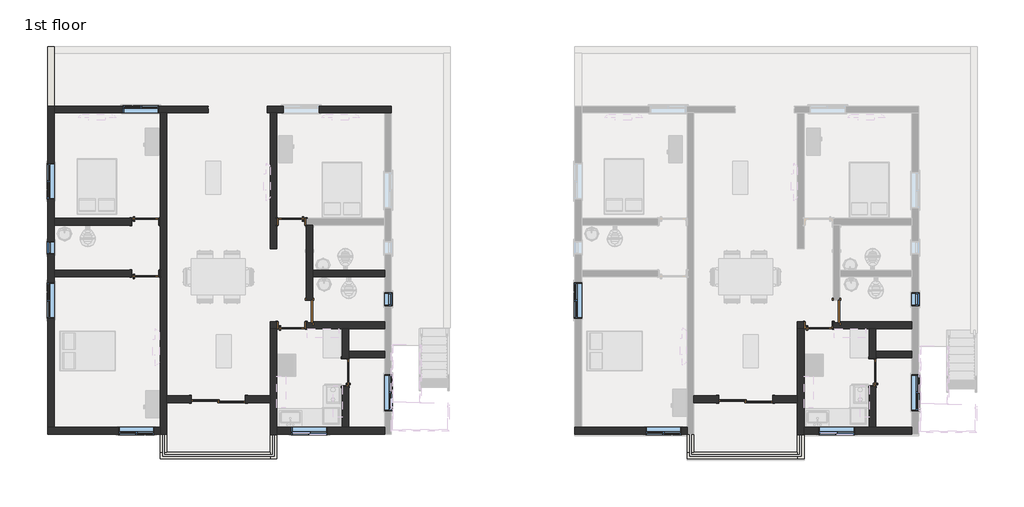
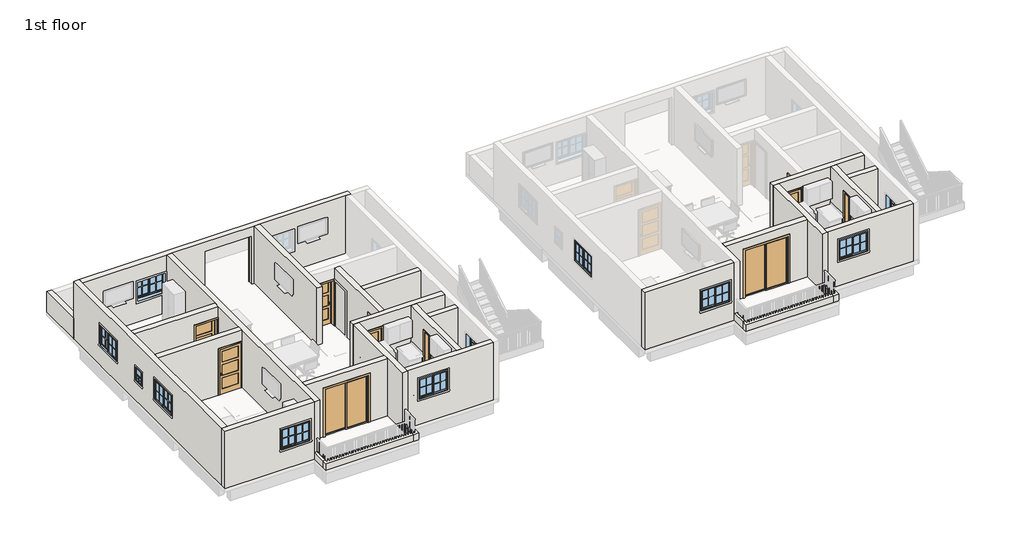
# One storey, part 1 of 8: 30 walls, 13 windows, 11 doors.
"""IFC4 building model written with IfcOpenShell, lengths in millimetres."""

from ifc_helpers import new_model, si_unit, frame, origin, place, context, project, spatial, polyline, outline, extrude, faceted_brep, transform, mapped, element, save
from components import door_d4d75d1e, door_2334f446, door_80766924, door_a1484949, window_608ea798, window_2eef0573, window_a5b1ea32

model = new_model("IFC4")

# Units and contexts
model_context = context("Model", 3, world=origin())
ifc_project = project(units=[si_unit("LENGTHUNIT", "METRE", prefix="MILLI")], contexts=[model_context])

# Site, building, storey
site = spatial("IfcSite", under=ifc_project)
building = spatial("IfcBuilding", under=site)
storey = spatial("IfcBuildingStorey", under=building, Name="1st floor", Elevation=3810.0)

# Doors
placement = place(None, origin())
door_shape = door_d4d75d1e(model_context)
element("IfcDoor", 1, ObjectType="Door-Double-Sliding : 72\" x 84\"", at=placement, inside=storey, context=model_context, shape_type="MappedRepresentation", body=[
    mapped(door_shape, transform((-10509.3993763, -3297.2064015, 3810.0), x_axis=(-1.0, 0.0, 0.0), y_axis=(0.0, -1.0, 0.0), z_axis=(0.0, 0.0, 1.0))),
])
element("IfcDoor", 2, ObjectType="Door-Double-Sliding : 72\" x 84\"", at=placement, inside=storey, context=model_context, shape_type="MappedRepresentation", body=[
    mapped(door_shape, transform((7365.1761273, -3297.2064015, 3810.0), x_axis=(-1.0, 0.0, 0.0), y_axis=(0.0, -1.0, 0.0), z_axis=(0.0, 0.0, 1.0))),
])
door_2_shape = door_2334f446(model_context)
element("IfcDoor", 3, ObjectType="Door-Interior-Single-3_Panel_Vert-Wood : 36\" x 80\"", at=placement, inside=storey, context=model_context, shape_type="MappedRepresentation", body=[
    mapped(door_2_shape, transform((-12985.8993763, 2598.7685985, 3810.0), x_axis=(1.0, 0.0, 0.0), y_axis=(0.0, 1.0, 0.0), z_axis=(0.0, 0.0, 1.0))),
])
door_3_shape = door_80766924(model_context)
element("IfcDoor", 4, ObjectType="Door-Interior-Single-3_Panel_Vert-Wood : 36\" x 80\"", at=placement, inside=storey, context=model_context, shape_type="MappedRepresentation", body=[
    mapped(door_3_shape, transform((-12985.8993763, 839.8185985, 3810.0), x_axis=(1.0, 0.0, 0.0), y_axis=(0.0, 1.0, 0.0), z_axis=(0.0, 0.0, 1.0))),
])
element("IfcDoor", 5, ObjectType="Door-Interior-Single-3_Panel_Vert-Wood : 36\" x 80\"", at=placement, inside=storey, context=model_context, shape_type="MappedRepresentation", body=[
    mapped(door_3_shape, transform((-6200.9243763, -2509.8064015, 3810.0), x_axis=(0.0, 1.0, 0.0), y_axis=(-1.0, 0.0, 0.0), z_axis=(0.0, 0.0, 1.0))),
])
element("IfcDoor", 6, ObjectType="Door-Interior-Single-3_Panel_Vert-Wood : 36\" x 80\"", at=placement, inside=storey, context=model_context, shape_type="MappedRepresentation", body=[
    mapped(door_3_shape, transform((-8032.8993763, -912.7814015, 3810.0), x_axis=(1.0, 0.0, 0.0), y_axis=(0.0, 1.0, 0.0), z_axis=(0.0, 0.0, 1.0))),
])
element("IfcDoor", 7, ObjectType="Door-Interior-Single-3_Panel_Vert-Wood : 36\" x 80\"", at=placement, inside=storey, context=model_context, shape_type="MappedRepresentation", body=[
    mapped(door_3_shape, transform((-8032.8993763, 2598.7685985, 3810.0), x_axis=(-1.0, 0.0, 0.0), y_axis=(0.0, -1.0, 0.0), z_axis=(0.0, 0.0, 1.0))),
])
element("IfcDoor", 8, ObjectType="Door-Interior-Single-3_Panel_Vert-Wood : 36\" x 80\"", at=placement, inside=storey, context=model_context, shape_type="MappedRepresentation", body=[
    mapped(door_3_shape, transform((11673.6511273, -2509.8064015, 3810.0), x_axis=(0.0, 1.0, 0.0), y_axis=(-1.0, 0.0, 0.0), z_axis=(0.0, 0.0, 1.0))),
])
element("IfcDoor", 9, ObjectType="Door-Interior-Single-3_Panel_Vert-Wood : 36\" x 80\"", at=placement, inside=storey, context=model_context, shape_type="MappedRepresentation", body=[
    mapped(door_3_shape, transform((9841.6761273, -912.7814015, 3810.0), x_axis=(1.0, 0.0, 0.0), y_axis=(0.0, 1.0, 0.0), z_axis=(0.0, 0.0, 1.0))),
])
door_4_shape = door_a1484949(model_context)
element("IfcDoor", 10, ObjectType="Single-Flush : 30\" x 80\"", at=placement, inside=storey, context=model_context, shape_type="MappedRepresentation", body=[
    mapped(door_4_shape, transform((-7423.2993763, -452.4064015, 3810.0), x_axis=(0.0, -1.0, 0.0), y_axis=(1.0, 0.0, 0.0), z_axis=(0.0, 0.0, 1.0))),
])
element("IfcDoor", 11, ObjectType="Single-Flush : 30\" x 80\"", at=placement, inside=storey, context=model_context, shape_type="MappedRepresentation", body=[
    mapped(door_4_shape, transform((10451.2761273, -452.4064015, 3810.0), x_axis=(0.0, -1.0, 0.0), y_axis=(1.0, 0.0, 0.0), z_axis=(0.0, 0.0, 1.0))),
])

# Walls
element("IfcWall", 12, at=placement, inside=storey, context=model_context, shape_type="Brep", body=[
    faceted_brep([(-16300.5993763, 6519.8935985, 3810.0), (-16300.5993763, -4376.7064015, 3810.0), (-16300.5993763, -4376.7064015, 6400.8), (-16300.5993763, 6519.8935985, 6400.8), (-16300.5993763, 4576.7935985, 5638.8), (-16300.5993763, 3357.5935985, 5638.8), (-16300.5993763, 3357.5935985, 4724.4), (-16300.5993763, 4576.7935985, 4724.4), (-16300.5993763, -681.0064015, 5638.8), (-16300.5993763, -681.0064015, 4724.4), (-16300.5993763, 538.1935985, 4724.4), (-16300.5993763, 538.1935985, 5638.8), (-16300.5993763, 1935.1935985, 5334.0), (-16300.5993763, 1503.3935985, 5334.0), (-16300.5993763, 1503.3935985, 4724.4), (-16300.5993763, 1935.1935985, 4724.4), (-16071.9993763, 6519.8935985, 3810.0), (-16071.9993763, 6519.8935985, 6400.8), (-16071.9993763, 6291.2935985, 6400.8), (-16071.9993763, 2709.8935985, 6400.8), (-16071.9993763, 2481.2935985, 6400.8), (-16071.9993763, 957.2935985, 6400.8), (-16071.9993763, 728.6935985, 6400.8), (-16071.9993763, -4376.7064015, 6400.8), (-16071.9993763, -4376.7064015, 3810.0), (-16071.9993763, 728.6935985, 3810.0), (-16071.9993763, 957.2935985, 3810.0), (-16071.9993763, 2481.2935985, 3810.0), (-16071.9993763, 2709.8935985, 3810.0), (-16071.9993763, 6291.2935985, 3810.0), (-16071.9993763, 4576.7935985, 5638.8), (-16071.9993763, 4576.7935985, 4724.4), (-16071.9993763, 3357.5935985, 4724.4), (-16071.9993763, 3357.5935985, 5638.8), (-16071.9993763, -681.0064015, 5638.8), (-16071.9993763, 538.1935985, 5638.8), (-16071.9993763, 538.1935985, 4724.4), (-16071.9993763, -681.0064015, 4724.4), (-16071.9993763, 1935.1935985, 5334.0), (-16071.9993763, 1935.1935985, 4724.4), (-16071.9993763, 1503.3935985, 4724.4), (-16071.9993763, 1503.3935985, 5334.0)], [[[0, 1, 2, 3], [4, 5, 6, 7], [8, 9, 10, 11], [12, 13, 14, 15]], [[16, 17, 18, 19, 20, 21, 22, 23, 24, 25, 26, 27, 28, 29], [30, 31, 32, 33], [34, 35, 36, 37], [38, 39, 40, 41]], [[1, 0, 16, 29, 28, 27, 26, 25, 24]], [[3, 2, 23, 22, 21, 20, 19, 18, 17]], [[0, 3, 17, 16]], [[2, 1, 24, 23]], [[31, 30, 4, 7]], [[32, 31, 7, 6]], [[33, 32, 6, 5]], [[30, 33, 5, 4]], [[9, 8, 34, 37]], [[10, 9, 37, 36]], [[11, 10, 36, 35]], [[8, 11, 35, 34]], [[39, 38, 12, 15]], [[40, 39, 15, 14]], [[41, 40, 14, 13]], [[38, 41, 13, 12]]]),
])
element("IfcWall", 13, at=placement, inside=storey, context=model_context, shape_type="SweptSolid", body=[
    extrude(outline(polyline([(6400.8, -12490.5993763), (6400.8, -16071.9993763), (3810.0, -16071.9993763), (3810.0, -13468.4993763), (5867.4, -13468.4993763), (5867.4, -12503.2993763), (3810.0, -12503.2993763), (3810.0, -12490.5993763), (6400.8, -12490.5993763)])), frame((0.0, 2481.2935985, 0.0), z_axis=(0.0, 1.0, 0.0), x_axis=(0.0, 0.0, 1.0)), (0.0, 0.0, 1.0), 228.6),
])
element("IfcWall", 14, at=placement, inside=storey, context=model_context, shape_type="Brep", body=[
    faceted_brep([(-4641.9993763, 6291.2935985, 6400.8), (-4870.5993763, 6291.2935985, 6400.8), (-8528.1993763, 6291.2935985, 6400.8), (-8756.7993763, 6291.2935985, 6400.8), (-12261.9993763, 6291.2935985, 6400.8), (-12490.5993763, 6291.2935985, 6400.8), (-16071.9993763, 6291.2935985, 6400.8), (-16071.9993763, 6291.2935985, 3810.0), (-12490.5993763, 6291.2935985, 3810.0), (-12261.9993763, 6291.2935985, 3810.0), (-10861.6993763, 6291.2935985, 3810.0), (-10861.6993763, 6291.2935985, 5979.5), (-8861.6993763, 6291.2935985, 5979.5), (-8861.6993763, 6291.2935985, 3810.0), (-8756.7993763, 6291.2935985, 3810.0), (-8528.1993763, 6291.2935985, 3810.0), (-4870.5993763, 6291.2935985, 3810.0), (-4641.9993763, 6291.2935985, 3810.0), (-8312.2993763, 6291.2935985, 5638.8), (-7093.0993763, 6291.2935985, 5638.8), (-7093.0993763, 6291.2935985, 4724.4), (-8312.2993763, 6291.2935985, 4724.4), (-12528.6993763, 6291.2935985, 5638.8), (-12528.6993763, 6291.2935985, 4724.4), (-13747.8993763, 6291.2935985, 4724.4), (-13747.8993763, 6291.2935985, 5638.8), (-16071.9993763, 6519.8935985, 6400.8), (-4641.9993763, 6519.8935985, 6400.8), (-4641.9993763, 6519.8935985, 3810.0), (-8861.6993763, 6519.8935985, 3810.0), (-8861.6993763, 6519.8935985, 5979.5), (-10861.6993763, 6519.8935985, 5979.5), (-10861.6993763, 6519.8935985, 3810.0), (-16071.9993763, 6519.8935985, 3810.0), (-8312.2993763, 6519.8935985, 5638.8), (-8312.2993763, 6519.8935985, 4724.4), (-7093.0993763, 6519.8935985, 4724.4), (-7093.0993763, 6519.8935985, 5638.8), (-12528.6993763, 6519.8935985, 5638.8), (-13747.8993763, 6519.8935985, 5638.8), (-13747.8993763, 6519.8935985, 4724.4), (-12528.6993763, 6519.8935985, 4724.4), (-10861.6993763, 6499.8935985, 3810.0), (-10876.6993763, 6499.8935985, 3810.0), (-10876.6993763, 6429.8935985, 3810.0), (-10861.6993763, 6429.8935985, 3810.0), (-8861.6993763, 6429.8935985, 3810.0), (-8846.6993763, 6429.8935985, 3810.0), (-8846.6993763, 6499.8935985, 3810.0), (-8861.6993763, 6499.8935985, 3810.0), (-8861.6993763, 6499.8935985, 5979.5), (-10861.6993763, 6499.8935985, 5979.5), (-10861.6993763, 6429.8935985, 5979.5), (-8861.6993763, 6429.8935985, 5979.5), (-10876.6993763, 6429.8935985, 5994.5), (-8846.6993763, 6429.8935985, 5994.5), (-8846.6993763, 6499.8935985, 5994.5), (-10876.6993763, 6499.8935985, 5994.5)], [[[0, 1, 2, 3, 4, 5, 6, 7, 8, 9, 10, 11, 12, 13, 14, 15, 16, 17], [18, 19, 20, 21], [22, 23, 24, 25]], [[26, 27, 28, 29, 30, 31, 32, 33], [34, 35, 36, 37], [38, 39, 40, 41]], [[7, 33, 32, 42, 43, 44, 45, 10, 9, 8]], [[28, 17, 16, 15, 14, 13, 46, 47, 48, 49, 29]], [[6, 5, 4, 3, 2, 1, 0, 27, 26]], [[7, 6, 26, 33]], [[0, 17, 28, 27]], [[50, 51, 31, 30]], [[52, 53, 12, 11]], [[45, 52, 11, 10]], [[53, 46, 13, 12]], [[53, 52, 45, 44, 54, 55, 47, 46]], [[47, 55, 56, 48]], [[51, 50, 49, 48, 56, 57, 43, 42]], [[49, 50, 30, 29]], [[51, 42, 32, 31]], [[54, 44, 43, 57]], [[55, 54, 57, 56]], [[35, 34, 18, 21]], [[36, 35, 21, 20]], [[37, 36, 20, 19]], [[34, 37, 19, 18]], [[23, 22, 38, 41]], [[24, 23, 41, 40]], [[25, 24, 40, 39]], [[22, 25, 39, 38]]]),
])
element("IfcWall", 15, at=placement, inside=storey, context=model_context, shape_type="Brep", body=[
    faceted_brep([(-4870.5993763, -4376.7064015, 3810.0), (-6089.7993763, -4376.7064015, 3810.0), (-6318.3993763, -4376.7064015, 3810.0), (-8528.1993763, -4376.7064015, 3810.0), (-8528.1993763, -4376.7064015, 6400.8), (-6318.3993763, -4376.7064015, 6400.8), (-6089.7993763, -4376.7064015, 6400.8), (-4870.5993763, -4376.7064015, 6400.8), (-8032.8993763, -4376.7064015, 5867.4), (-8032.8993763, -4376.7064015, 4953.0), (-6813.6993763, -4376.7064015, 4953.0), (-6813.6993763, -4376.7064015, 5867.4), (-4870.5993763, -4605.3064015, 3810.0), (-4870.5993763, -4605.3064015, 6400.8), (-8528.1993763, -4605.3064015, 6400.8), (-8528.1993763, -4605.3064015, 3810.0), (-8032.8993763, -4605.3064015, 5867.4), (-6813.6993763, -4605.3064015, 5867.4), (-6813.6993763, -4605.3064015, 4953.0), (-8032.8993763, -4605.3064015, 4953.0)], [[[0, 1, 2, 3, 4, 5, 6, 7], [8, 9, 10, 11]], [[12, 13, 14, 15], [16, 17, 18, 19]], [[3, 2, 1, 0, 12, 15]], [[7, 6, 5, 4, 14, 13]], [[0, 7, 13, 12]], [[4, 3, 15, 14]], [[9, 8, 16, 19]], [[10, 9, 19, 18]], [[11, 10, 18, 17]], [[8, 11, 17, 16]]]),
])
element("IfcWall", 16, at=placement, inside=storey, context=model_context, shape_type="Brep", body=[
    faceted_brep([(-8756.7993763, 6291.2935985, 3810.0), (-8756.7993763, 1681.1935985, 3810.0), (-8756.7993763, 1681.1935985, 6400.8), (-8756.7993763, 6291.2935985, 6400.8), (-8528.1993763, 6291.2935985, 3810.0), (-8528.1993763, 6291.2935985, 6400.8), (-8528.1993763, 2709.8935985, 6400.8), (-8528.1993763, 2481.2935985, 6400.8), (-8528.1993763, 1681.1935985, 6400.8), (-8528.1993763, 1681.1935985, 3810.0), (-8528.1993763, 2481.2935985, 3810.0), (-8528.1993763, 2709.8935985, 3810.0)], [[[0, 1, 2, 3]], [[4, 5, 6, 7, 8, 9, 10, 11]], [[1, 0, 4, 11, 10, 9]], [[2, 1, 9, 8]], [[3, 2, 8, 7, 6, 5]], [[0, 3, 5, 4]]]),
])
element("IfcWall", 17, at=placement, inside=storey, context=model_context, shape_type="Brep", body=[
    faceted_brep([(-8756.7993763, -5214.9064015, 3810.0), (-12261.9993763, -5214.9064015, 3810.0), (-12490.5993763, -5214.9064015, 3810.0), (-12490.5993763, -5214.9064015, 4114.8), (-12261.9993763, -5214.9064015, 4114.8), (-8756.7993763, -5214.9064015, 4114.8), (-8756.7993763, -5443.5064015, 3810.0), (-8756.7993763, -5443.5064015, 4114.8), (-12490.5993763, -5443.5064015, 4114.8), (-12490.5993763, -5443.5064015, 3810.0)], [[[0, 1, 2, 3, 4, 5]], [[6, 7, 8, 9]], [[2, 1, 0, 6, 9]], [[5, 4, 3, 8, 7]], [[0, 5, 7, 6]], [[3, 2, 9, 8]]]),
])
element("IfcWall", 18, at=placement, inside=storey, context=model_context, shape_type="SweptSolid", body=[
    extrude(outline(polyline([(-12261.9993763, -4611.6564015), (-12261.9993763, -5214.9064015), (-12490.5993763, -5214.9064015), (-12490.5993763, -4611.6564015), (-12261.9993763, -4611.6564015)])), frame((0.0, 0.0, 3810.0), z_axis=(0.0, 0.0, 1.0), x_axis=(1.0, 0.0, 0.0)), (0.0, 0.0, 1.0), 304.8),
])
element("IfcWall", 19, at=placement, inside=storey, context=model_context, shape_type="Brep", body=[
    faceted_brep([(-16300.5993763, -4605.3064015, 3810.0), (-12490.5993763, -4605.3064015, 3810.0), (-12490.5993763, -4605.3064015, 6400.8), (-16300.5993763, -4605.3064015, 6400.8), (-13900.2993763, -4605.3064015, 5638.8), (-12681.0993763, -4605.3064015, 5638.8), (-12681.0993763, -4605.3064015, 4724.4), (-13900.2993763, -4605.3064015, 4724.4), (-16300.5993763, -4376.7064015, 3810.0), (-16300.5993763, -4376.7064015, 6400.8), (-16071.9993763, -4376.7064015, 6400.8), (-12490.5993763, -4376.7064015, 6400.8), (-12490.5993763, -4376.7064015, 3810.0), (-16071.9993763, -4376.7064015, 3810.0), (-13900.2993763, -4376.7064015, 5638.8), (-13900.2993763, -4376.7064015, 4724.4), (-12681.0993763, -4376.7064015, 4724.4), (-12681.0993763, -4376.7064015, 5638.8)], [[[0, 1, 2, 3], [4, 5, 6, 7]], [[8, 9, 10, 11, 12, 13], [14, 15, 16, 17]], [[1, 0, 8, 13, 12]], [[3, 2, 11, 10, 9]], [[0, 3, 9, 8]], [[15, 14, 4, 7]], [[16, 15, 7, 6]], [[17, 16, 6, 5]], [[14, 17, 5, 4]], [[2, 1, 12, 11]]]),
])
element("IfcWall", 20, at=placement, inside=storey, context=model_context, shape_type="SweptSolid", body=[
    extrude(outline(polyline([(3810.0, -12261.9993763), (3810.0, -11423.7993763), (5943.6, -11423.7993763), (5943.6, -9594.9993763), (3810.0, -9594.9993763), (3810.0, -8756.7993763), (6400.8, -8756.7993763), (6400.8, -12261.9993763), (3810.0, -12261.9993763)])), frame((0.0, -3538.5064015, 0.0), z_axis=(0.0, 1.0, 0.0), x_axis=(0.0, 0.0, 1.0)), (0.0, 0.0, 1.0), 228.6),
])
element("IfcWall", 21, at=placement, inside=storey, context=model_context, shape_type="Brep", body=[
    faceted_brep([(-8756.7993763, -795.3064015, 6400.8), (-7537.5993763, -795.3064015, 6400.8), (-7308.9993763, -795.3064015, 6400.8), (-4870.5993763, -795.3064015, 6400.8), (-4870.5993763, -795.3064015, 3810.0), (-7308.9993763, -795.3064015, 3810.0), (-7308.9993763, -795.3064015, 5842.0), (-7537.5993763, -795.3064015, 5842.0), (-7537.5993763, -795.3064015, 3810.0), (-7550.2993763, -795.3064015, 3810.0), (-7550.2993763, -795.3064015, 5867.4), (-8515.4993763, -795.3064015, 5867.4), (-8515.4993763, -795.3064015, 3810.0), (-8756.7993763, -795.3064015, 3810.0), (-4870.5993763, -1023.9064015, 6400.8), (-6089.7993763, -1023.9064015, 6400.8), (-6318.3993763, -1023.9064015, 6400.8), (-8528.1993763, -1023.9064015, 6400.8), (-8756.7993763, -1023.9064015, 6400.8), (-8756.7993763, -1023.9064015, 3810.0), (-8528.1993763, -1023.9064015, 3810.0), (-8515.4993763, -1023.9064015, 3810.0), (-8515.4993763, -1023.9064015, 5867.4), (-7550.2993763, -1023.9064015, 5867.4), (-7550.2993763, -1023.9064015, 3810.0), (-6318.3993763, -1023.9064015, 3810.0), (-6089.7993763, -1023.9064015, 3810.0), (-4870.5993763, -1023.9064015, 3810.0), (-7537.5993763, -833.4064015, 3810.0), (-7308.9993763, -833.4064015, 3810.0), (-7537.5993763, -833.4064015, 5842.0), (-7308.9993763, -833.4064015, 5842.0)], [[[0, 1, 2, 3, 4, 5, 6, 7, 8, 9, 10, 11, 12, 13]], [[14, 15, 16, 17, 18, 19, 20, 21, 22, 23, 24, 25, 26, 27]], [[4, 27, 26, 25, 24, 9, 8, 28, 29, 5]], [[13, 12, 21, 20, 19]], [[3, 2, 1, 0, 18, 17, 16, 15, 14]], [[4, 3, 14, 27]], [[23, 10, 9, 24]], [[10, 23, 22, 11]], [[11, 22, 21, 12]], [[30, 28, 8, 7]], [[29, 31, 6, 5]], [[28, 30, 31, 29]], [[31, 30, 7, 6]], [[0, 13, 19, 18]]]),
])
element("IfcWall", 22, at=placement, inside=storey, context=model_context, shape_type="Brep", body=[
    faceted_brep([(-6318.3993763, -4376.7064015, 6400.8), (-6318.3993763, -1023.9064015, 6400.8), (-6318.3993763, -1023.9064015, 3810.0), (-6318.3993763, -2027.2064015, 3810.0), (-6318.3993763, -2027.2064015, 5867.4), (-6318.3993763, -2992.4064015, 5867.4), (-6318.3993763, -2992.4064015, 3810.0), (-6318.3993763, -4376.7064015, 3810.0), (-6089.7993763, -1023.9064015, 6400.8), (-6089.7993763, -1785.9064015, 6400.8), (-6089.7993763, -2014.5064015, 6400.8), (-6089.7993763, -4376.7064015, 6400.8), (-6089.7993763, -4376.7064015, 3810.0), (-6089.7993763, -2992.4064015, 3810.0), (-6089.7993763, -2992.4064015, 5867.4), (-6089.7993763, -2027.2064015, 5867.4), (-6089.7993763, -2027.2064015, 3810.0), (-6089.7993763, -2014.5064015, 3810.0), (-6089.7993763, -1785.9064015, 3810.0), (-6089.7993763, -1023.9064015, 3810.0)], [[[0, 1, 2, 3, 4, 5, 6, 7]], [[8, 9, 10, 11, 12, 13, 14, 15, 16, 17, 18, 19]], [[2, 19, 18, 17, 16, 3]], [[12, 7, 6, 13]], [[1, 0, 11, 10, 9, 8]], [[2, 1, 8, 19]], [[0, 7, 12, 11]], [[15, 4, 3, 16]], [[4, 15, 14, 5]], [[5, 14, 13, 6]]]),
])
element("IfcWall", 23, at=placement, inside=storey, context=model_context, shape_type="SweptSolid", body=[
    extrude(outline(polyline([(-4870.5993763, -2014.5064015), (-6089.7993763, -2014.5064015), (-6089.7993763, -1785.9064015), (-4870.5993763, -1785.9064015), (-4870.5993763, -2014.5064015)])), frame((0.0, 0.0, 3810.0), z_axis=(0.0, 0.0, 1.0), x_axis=(1.0, 0.0, 0.0)), (0.0, 0.0, 1.0), 2590.8),
])
element("IfcWall", 24, at=placement, inside=storey, context=model_context, shape_type="SweptSolid", body=[
    extrude(outline(polyline([(-7308.9993763, 957.2935985), (-4870.5993763, 957.2935985), (-4870.5993763, 728.6935985), (-7308.9993763, 728.6935985), (-7308.9993763, 957.2935985)])), frame((0.0, 0.0, 3810.0), z_axis=(0.0, 0.0, 1.0), x_axis=(1.0, 0.0, 0.0)), (0.0, 0.0, 1.0), 2590.8),
])
element("IfcWall", 25, at=placement, inside=storey, context=model_context, shape_type="Brep", body=[
    faceted_brep([(-7308.9993763, 2481.2935985, 6400.8), (-7308.9993763, 957.2935985, 6400.8), (-7308.9993763, 728.6935985, 6400.8), (-7308.9993763, -795.3064015, 6400.8), (-7308.9993763, -795.3064015, 5842.0), (-7308.9993763, -71.4064015, 5842.0), (-7308.9993763, -71.4064015, 3810.0), (-7308.9993763, 728.6935985, 3810.0), (-7308.9993763, 957.2935985, 3810.0), (-7308.9993763, 2481.2935985, 3810.0), (-7537.5993763, -795.3064015, 6400.8), (-7537.5993763, 2481.2935985, 6400.8), (-7537.5993763, 2481.2935985, 3810.0), (-7537.5993763, -71.4064015, 3810.0), (-7537.5993763, -71.4064015, 5842.0), (-7537.5993763, -795.3064015, 5842.0)], [[[0, 1, 2, 3, 4, 5, 6, 7, 8, 9]], [[10, 11, 12, 13, 14, 15]], [[12, 9, 8, 7, 6, 13]], [[3, 2, 1, 0, 11, 10]], [[3, 10, 15, 4]], [[0, 9, 12, 11]], [[14, 5, 4, 15]], [[5, 14, 13, 6]]]),
])
element("IfcWall", 26, at=placement, inside=storey, context=model_context, shape_type="SweptSolid", body=[
    extrude(outline(polyline([(2481.2935985, 3810.0), (2405.0935985, 3810.0), (2405.0935985, 5842.0), (1643.0935985, 5842.0), (1643.0935985, 3810.0), (957.2935985, 3810.0), (957.2935985, 6400.8), (2481.2935985, 6400.8), (2481.2935985, 3810.0)])), frame((-7537.5993763, 0.0, 0.0), z_axis=(1.0, 0.0, 0.0), x_axis=(0.0, 1.0, 0.0)), (0.0, 0.0, 1.0), 228.6),
])
element("IfcWall", 27, at=placement, inside=storey, context=model_context, shape_type="SweptSolid", body=[
    extrude(outline(polyline([(6400.8, -12490.5993763), (6400.8, -16071.9993763), (3810.0, -16071.9993763), (3810.0, -13468.4993763), (5867.4, -13468.4993763), (5867.4, -12503.2993763), (3810.0, -12503.2993763), (3810.0, -12490.5993763), (6400.8, -12490.5993763)])), frame((0.0, 728.6935985, 0.0), z_axis=(0.0, 1.0, 0.0), x_axis=(0.0, 0.0, 1.0)), (0.0, 0.0, 1.0), 228.6),
])
element("IfcWall", 28, at=placement, inside=storey, context=model_context, shape_type="Brep", body=[
    faceted_brep([(-8756.7993763, -1023.9064015, 3810.0), (-8756.7993763, -3309.9064015, 3810.0), (-8756.7993763, -3538.5064015, 3810.0), (-8756.7993763, -4618.0064015, 3810.0), (-8756.7993763, -4618.0064015, 4114.8), (-8756.7993763, -4618.0064015, 6400.8), (-8756.7993763, -3538.5064015, 6400.8), (-8756.7993763, -3309.9064015, 6400.8), (-8756.7993763, -1023.9064015, 6400.8), (-8528.1993763, -1023.9064015, 3810.0), (-8528.1993763, -1023.9064015, 6400.8), (-8528.1993763, -4376.7064015, 6400.8), (-8528.1993763, -4605.3064015, 6400.8), (-8528.1993763, -4618.0064015, 6400.8), (-8528.1993763, -4618.0064015, 4114.8), (-8528.1993763, -4618.0064015, 3810.0), (-8528.1993763, -4605.3064015, 3810.0), (-8528.1993763, -4376.7064015, 3810.0)], [[[0, 1, 2, 3, 4, 5, 6, 7, 8]], [[9, 10, 11, 12, 13, 14, 15, 16, 17]], [[3, 2, 1, 0, 9, 17, 16, 15]], [[5, 4, 3, 15, 14, 13]], [[8, 7, 6, 5, 13, 12, 11, 10]], [[0, 8, 10, 9]]]),
])
element("IfcWall", 29, at=placement, inside=storey, context=model_context, shape_type="Brep", body=[
    faceted_brep([(-12261.9993763, -4605.3064015, 3810.0), (-12261.9993763, -3538.5064015, 3810.0), (-12261.9993763, -3309.9064015, 3810.0), (-12261.9993763, 6291.2935985, 3810.0), (-12261.9993763, 6291.2935985, 6400.8), (-12261.9993763, -3309.9064015, 6400.8), (-12261.9993763, -3538.5064015, 6400.8), (-12261.9993763, -4605.3064015, 6400.8), (-12490.5993763, -4605.3064015, 3810.0), (-12490.5993763, -4605.3064015, 6400.8), (-12490.5993763, -4376.7064015, 6400.8), (-12490.5993763, 728.6935985, 6400.8), (-12490.5993763, 957.2935985, 6400.8), (-12490.5993763, 2481.2935985, 6400.8), (-12490.5993763, 2709.8935985, 6400.8), (-12490.5993763, 6291.2935985, 6400.8), (-12490.5993763, 6291.2935985, 3810.0), (-12490.5993763, 2709.8935985, 3810.0), (-12490.5993763, 2481.2935985, 3810.0), (-12490.5993763, 957.2935985, 3810.0), (-12490.5993763, 728.6935985, 3810.0), (-12490.5993763, -4376.7064015, 3810.0)], [[[0, 1, 2, 3, 4, 5, 6, 7]], [[8, 9, 10, 11, 12, 13, 14, 15, 16, 17, 18, 19, 20, 21]], [[3, 2, 1, 0, 8, 21, 20, 19, 18, 17, 16]], [[7, 6, 5, 4, 15, 14, 13, 12, 11, 10, 9]], [[4, 3, 16, 15]], [[0, 7, 9, 8]]]),
])
element("IfcWall", 30, at=placement, inside=storey, context=model_context, shape_type="Brep", body=[
    faceted_brep([(-8756.7993763, -4618.0064015, 3810.0), (-8756.7993763, -5214.9064015, 3810.0), (-8756.7993763, -5443.5064015, 3810.0), (-8756.7993763, -5443.5064015, 4114.8), (-8756.7993763, -5214.9064015, 4114.8), (-8756.7993763, -4618.0064015, 4114.8), (-8528.1993763, -4618.0064015, 3810.0), (-8528.1993763, -4618.0064015, 4114.8), (-8528.1993763, -5443.5064015, 4114.8), (-8528.1993763, -5443.5064015, 3810.0)], [[[0, 1, 2, 3, 4, 5]], [[6, 7, 8, 9]], [[2, 1, 0, 6, 9]], [[5, 4, 3, 8, 7]], [[0, 5, 7, 6]], [[3, 2, 9, 8]]]),
])
element("IfcWall", 31, at=placement, inside=storey, context=model_context, shape_type="Brep", body=[
    faceted_brep([(13003.9761273, -4376.7064015, 3810.0), (11784.7761273, -4376.7064015, 3810.0), (11556.1761273, -4376.7064015, 3810.0), (9346.3761273, -4376.7064015, 3810.0), (9346.3761273, -4376.7064015, 6400.8), (11556.1761273, -4376.7064015, 6400.8), (11784.7761273, -4376.7064015, 6400.8), (13003.9761273, -4376.7064015, 6400.8), (9841.6761273, -4376.7064015, 5867.4), (9841.6761273, -4376.7064015, 4953.0), (11060.8761273, -4376.7064015, 4953.0), (11060.8761273, -4376.7064015, 5867.4), (13003.9761273, -4605.3064015, 3810.0), (13003.9761273, -4605.3064015, 6400.8), (9346.3761273, -4605.3064015, 6400.8), (9346.3761273, -4605.3064015, 3810.0), (9841.6761273, -4605.3064015, 5867.4), (11060.8761273, -4605.3064015, 5867.4), (11060.8761273, -4605.3064015, 4953.0), (9841.6761273, -4605.3064015, 4953.0)], [[[0, 1, 2, 3, 4, 5, 6, 7], [8, 9, 10, 11]], [[12, 13, 14, 15], [16, 17, 18, 19]], [[3, 2, 1, 0, 12, 15]], [[7, 6, 5, 4, 14, 13]], [[0, 7, 13, 12]], [[4, 3, 15, 14]], [[9, 8, 16, 19]], [[10, 9, 19, 18]], [[11, 10, 18, 17]], [[8, 11, 17, 16]]]),
])
element("IfcWall", 32, at=placement, inside=storey, context=model_context, shape_type="Brep", body=[
    faceted_brep([(9117.7761273, -5214.9064015, 3810.0), (5612.5761273, -5214.9064015, 3810.0), (5383.9761273, -5214.9064015, 3810.0), (5383.9761273, -5214.9064015, 4114.8), (5612.5761273, -5214.9064015, 4114.8), (9117.7761273, -5214.9064015, 4114.8), (9117.7761273, -5443.5064015, 3810.0), (9117.7761273, -5443.5064015, 4114.8), (5383.9761273, -5443.5064015, 4114.8), (5383.9761273, -5443.5064015, 3810.0)], [[[0, 1, 2, 3, 4, 5]], [[6, 7, 8, 9]], [[2, 1, 0, 6, 9]], [[5, 4, 3, 8, 7]], [[0, 5, 7, 6]], [[3, 2, 9, 8]]]),
])
element("IfcWall", 33, at=placement, inside=storey, context=model_context, shape_type="SweptSolid", body=[
    extrude(outline(polyline([(5612.5761273, -4611.6564015), (5612.5761273, -5214.9064015), (5383.9761273, -5214.9064015), (5383.9761273, -4611.6564015), (5612.5761273, -4611.6564015)])), frame((0.0, 0.0, 3810.0), z_axis=(0.0, 0.0, 1.0), x_axis=(1.0, 0.0, 0.0)), (0.0, 0.0, 1.0), 304.8),
])
element("IfcWall", 34, at=placement, inside=storey, context=model_context, shape_type="Brep", body=[
    faceted_brep([(1573.9761273, -4605.3064015, 3810.0), (5383.9761273, -4605.3064015, 3810.0), (5383.9761273, -4605.3064015, 6400.8), (1573.9761273, -4605.3064015, 6400.8), (3974.2761273, -4605.3064015, 5638.8), (5193.4761273, -4605.3064015, 5638.8), (5193.4761273, -4605.3064015, 4724.4), (3974.2761273, -4605.3064015, 4724.4), (1573.9761273, -4376.7064015, 3810.0), (1573.9761273, -4376.7064015, 6400.8), (1802.5761273, -4376.7064015, 6400.8), (5383.9761273, -4376.7064015, 6400.8), (5383.9761273, -4376.7064015, 3810.0), (1802.5761273, -4376.7064015, 3810.0), (3974.2761273, -4376.7064015, 5638.8), (3974.2761273, -4376.7064015, 4724.4), (5193.4761273, -4376.7064015, 4724.4), (5193.4761273, -4376.7064015, 5638.8)], [[[0, 1, 2, 3], [4, 5, 6, 7]], [[8, 9, 10, 11, 12, 13], [14, 15, 16, 17]], [[1, 0, 8, 13, 12]], [[3, 2, 11, 10, 9]], [[0, 3, 9, 8]], [[15, 14, 4, 7]], [[16, 15, 7, 6]], [[17, 16, 6, 5]], [[14, 17, 5, 4]], [[2, 1, 12, 11]]]),
])
element("IfcWall", 35, at=placement, inside=storey, context=model_context, shape_type="SweptSolid", body=[
    extrude(outline(polyline([(3810.0, 5612.5761273), (3810.0, 6450.7761273), (5943.6, 6450.7761273), (5943.6, 8279.5761273), (3810.0, 8279.5761273), (3810.0, 9117.7761273), (6400.8, 9117.7761273), (6400.8, 5612.5761273), (3810.0, 5612.5761273)])), frame((0.0, -3538.5064015, 0.0), z_axis=(0.0, 1.0, 0.0), x_axis=(0.0, 0.0, 1.0)), (0.0, 0.0, 1.0), 228.6),
])
element("IfcWall", 36, at=placement, inside=storey, context=model_context, shape_type="Brep", body=[
    faceted_brep([(9117.7761273, -795.3064015, 6400.8), (10336.9761273, -795.3064015, 6400.8), (10565.5761273, -795.3064015, 6400.8), (13003.9761273, -795.3064015, 6400.8), (13003.9761273, -795.3064015, 3810.0), (10565.5761273, -795.3064015, 3810.0), (10565.5761273, -795.3064015, 5842.0), (10336.9761273, -795.3064015, 5842.0), (10336.9761273, -795.3064015, 3810.0), (10324.2761273, -795.3064015, 3810.0), (10324.2761273, -795.3064015, 5867.4), (9359.0761273, -795.3064015, 5867.4), (9359.0761273, -795.3064015, 3810.0), (9117.7761273, -795.3064015, 3810.0), (13003.9761273, -1023.9064015, 6400.8), (11784.7761273, -1023.9064015, 6400.8), (11556.1761273, -1023.9064015, 6400.8), (9346.3761273, -1023.9064015, 6400.8), (9117.7761273, -1023.9064015, 6400.8), (9117.7761273, -1023.9064015, 3810.0), (9346.3761273, -1023.9064015, 3810.0), (9359.0761273, -1023.9064015, 3810.0), (9359.0761273, -1023.9064015, 5867.4), (10324.2761273, -1023.9064015, 5867.4), (10324.2761273, -1023.9064015, 3810.0), (11556.1761273, -1023.9064015, 3810.0), (11784.7761273, -1023.9064015, 3810.0), (13003.9761273, -1023.9064015, 3810.0), (10336.9761273, -833.4064015, 3810.0), (10565.5761273, -833.4064015, 3810.0), (10336.9761273, -833.4064015, 5842.0), (10565.5761273, -833.4064015, 5842.0)], [[[0, 1, 2, 3, 4, 5, 6, 7, 8, 9, 10, 11, 12, 13]], [[14, 15, 16, 17, 18, 19, 20, 21, 22, 23, 24, 25, 26, 27]], [[4, 27, 26, 25, 24, 9, 8, 28, 29, 5]], [[13, 12, 21, 20, 19]], [[3, 2, 1, 0, 18, 17, 16, 15, 14]], [[4, 3, 14, 27]], [[23, 10, 9, 24]], [[10, 23, 22, 11]], [[11, 22, 21, 12]], [[30, 28, 8, 7]], [[29, 31, 6, 5]], [[28, 30, 31, 29]], [[31, 30, 7, 6]], [[0, 13, 19, 18]]]),
])
element("IfcWall", 37, at=placement, inside=storey, context=model_context, shape_type="Brep", body=[
    faceted_brep([(11556.1761273, -4376.7064015, 6400.8), (11556.1761273, -1023.9064015, 6400.8), (11556.1761273, -1023.9064015, 3810.0), (11556.1761273, -2027.2064015, 3810.0), (11556.1761273, -2027.2064015, 5867.4), (11556.1761273, -2992.4064015, 5867.4), (11556.1761273, -2992.4064015, 3810.0), (11556.1761273, -4376.7064015, 3810.0), (11784.7761273, -1023.9064015, 6400.8), (11784.7761273, -1785.9064015, 6400.8), (11784.7761273, -2014.5064015, 6400.8), (11784.7761273, -4376.7064015, 6400.8), (11784.7761273, -4376.7064015, 3810.0), (11784.7761273, -2992.4064015, 3810.0), (11784.7761273, -2992.4064015, 5867.4), (11784.7761273, -2027.2064015, 5867.4), (11784.7761273, -2027.2064015, 3810.0), (11784.7761273, -2014.5064015, 3810.0), (11784.7761273, -1785.9064015, 3810.0), (11784.7761273, -1023.9064015, 3810.0)], [[[0, 1, 2, 3, 4, 5, 6, 7]], [[8, 9, 10, 11, 12, 13, 14, 15, 16, 17, 18, 19]], [[2, 19, 18, 17, 16, 3]], [[12, 7, 6, 13]], [[1, 0, 11, 10, 9, 8]], [[2, 1, 8, 19]], [[0, 7, 12, 11]], [[15, 4, 3, 16]], [[4, 15, 14, 5]], [[5, 14, 13, 6]]]),
])
element("IfcWall", 38, at=placement, inside=storey, context=model_context, shape_type="SweptSolid", body=[
    extrude(outline(polyline([(13003.9761273, -2014.5064015), (11784.7761273, -2014.5064015), (11784.7761273, -1785.9064015), (13003.9761273, -1785.9064015), (13003.9761273, -2014.5064015)])), frame((0.0, 0.0, 3810.0), z_axis=(0.0, 0.0, 1.0), x_axis=(1.0, 0.0, 0.0)), (0.0, 0.0, 1.0), 2590.8),
])
element("IfcWall", 39, at=placement, inside=storey, context=model_context, shape_type="Brep", body=[
    faceted_brep([(9117.7761273, -1023.9064015, 3810.0), (9117.7761273, -3309.9064015, 3810.0), (9117.7761273, -3538.5064015, 3810.0), (9117.7761273, -4618.0064015, 3810.0), (9117.7761273, -4618.0064015, 4114.8), (9117.7761273, -4618.0064015, 6400.8), (9117.7761273, -3538.5064015, 6400.8), (9117.7761273, -3309.9064015, 6400.8), (9117.7761273, -1023.9064015, 6400.8), (9346.3761273, -1023.9064015, 3810.0), (9346.3761273, -1023.9064015, 6400.8), (9346.3761273, -4376.7064015, 6400.8), (9346.3761273, -4605.3064015, 6400.8), (9346.3761273, -4618.0064015, 6400.8), (9346.3761273, -4618.0064015, 4114.8), (9346.3761273, -4618.0064015, 3810.0), (9346.3761273, -4605.3064015, 3810.0), (9346.3761273, -4376.7064015, 3810.0)], [[[0, 1, 2, 3, 4, 5, 6, 7, 8]], [[9, 10, 11, 12, 13, 14, 15, 16, 17]], [[3, 2, 1, 0, 9, 17, 16, 15]], [[5, 4, 3, 15, 14, 13]], [[8, 7, 6, 5, 13, 12, 11, 10]], [[0, 8, 10, 9]]]),
])
element("IfcWall", 40, at=placement, inside=storey, context=model_context, shape_type="Brep", body=[
    faceted_brep([(9117.7761273, -4618.0064015, 3810.0), (9117.7761273, -5214.9064015, 3810.0), (9117.7761273, -5443.5064015, 3810.0), (9117.7761273, -5443.5064015, 4114.8), (9117.7761273, -5214.9064015, 4114.8), (9117.7761273, -4618.0064015, 4114.8), (9346.3761273, -4618.0064015, 3810.0), (9346.3761273, -4618.0064015, 4114.8), (9346.3761273, -5443.5064015, 4114.8), (9346.3761273, -5443.5064015, 3810.0)], [[[0, 1, 2, 3, 4, 5]], [[6, 7, 8, 9]], [[2, 1, 0, 6, 9]], [[5, 4, 3, 8, 7]], [[0, 5, 7, 6]], [[3, 2, 9, 8]]]),
])
element("IfcWall", 41, at=placement, inside=storey, context=model_context, shape_type="Brep", body=[
    faceted_brep([(-16071.9993763, 6526.2435985, 3810.0), (-16071.9993763, 8310.5935985, 3810.0), (-16071.9993763, 8539.1935985, 3810.0), (-16071.9993763, 8539.1935985, 4724.4), (-16071.9993763, 8310.5935985, 4724.4), (-16071.9993763, 6526.2435985, 4724.4), (-16300.5993763, 6526.2435985, 3810.0), (-16300.5993763, 6526.2435985, 4724.4), (-16300.5993763, 8539.1935985, 4724.4), (-16300.5993763, 8539.1935985, 3810.0)], [[[0, 1, 2, 3, 4, 5]], [[6, 7, 8, 9]], [[2, 1, 0, 6, 9]], [[5, 4, 3, 8, 7]], [[0, 5, 7, 6]], [[3, 2, 9, 8]]]),
])

# Windows
window_shape = window_608ea798(model_context)
element("IfcWindow", 42, ObjectType="Window-Fixed-Transom : 17\" x 24\"", at=placement, inside=storey, context=model_context, shape_type="MappedRepresentation", body=[
    mapped(window_shape, transform((-4756.2993763, -33.3064015, 3810.0), x_axis=(0.0, -1.0, 0.0), y_axis=(1.0, 0.0, 0.0), z_axis=(0.0, 0.0, 1.0))),
])
element("IfcWindow", 43, ObjectType="Window-Fixed-Transom : 17\" x 24\"", at=placement, inside=storey, context=model_context, shape_type="MappedRepresentation", body=[
    mapped(window_shape, transform((-16186.2993763, 1719.2935985, 3810.0), x_axis=(0.0, 1.0, 0.0), y_axis=(-1.0, 0.0, 0.0), z_axis=(0.0, 0.0, 1.0))),
])
element("IfcWindow", 44, ObjectType="Window-Fixed-Transom : 17\" x 24\"", at=placement, inside=storey, context=model_context, shape_type="MappedRepresentation", body=[
    mapped(window_shape, transform((13118.2761273, -33.3064015, 3810.0), x_axis=(0.0, -1.0, 0.0), y_axis=(1.0, 0.0, 0.0), z_axis=(0.0, 0.0, 1.0))),
])
window_2_shape = window_2eef0573(model_context)
element("IfcWindow", 45, ObjectType="Window-Sliding-Double : 48\" x 36\"", at=placement, inside=storey, context=model_context, shape_type="MappedRepresentation", body=[
    mapped(window_2_shape, transform((-7423.2993763, -4494.8164015, 4038.6), x_axis=(-1.0, 0.0, 0.0), y_axis=(0.0, -1.0, 0.0), z_axis=(0.0, 0.0, 1.0))),
])
element("IfcWindow", 46, ObjectType="Window-Sliding-Double : 48\" x 36\"", at=placement, inside=storey, context=model_context, shape_type="MappedRepresentation", body=[
    mapped(window_2_shape, transform((-13138.2993763, 6409.4035985, 3810.0), x_axis=(1.0, 0.0, 0.0), y_axis=(0.0, 1.0, 0.0), z_axis=(0.0, 0.0, 1.0))),
])
element("IfcWindow", 47, ObjectType="Window-Sliding-Double : 48\" x 36\"", at=placement, inside=storey, context=model_context, shape_type="MappedRepresentation", body=[
    mapped(window_2_shape, transform((-16190.1093763, 3967.1935985, 3810.0), x_axis=(0.0, 1.0, 0.0), y_axis=(-1.0, 0.0, 0.0), z_axis=(0.0, 0.0, 1.0))),
])
element("IfcWindow", 48, ObjectType="Window-Sliding-Double : 48\" x 36\"", at=placement, inside=storey, context=model_context, shape_type="MappedRepresentation", body=[
    mapped(window_2_shape, transform((-13290.6993763, -4494.8164015, 3810.0), x_axis=(-1.0, 0.0, 0.0), y_axis=(0.0, -1.0, 0.0), z_axis=(0.0, 0.0, 1.0))),
])
element("IfcWindow", 49, ObjectType="Window-Sliding-Double : 48\" x 36\"", at=placement, inside=storey, context=model_context, shape_type="MappedRepresentation", body=[
    mapped(window_2_shape, transform((-4752.4893763, -3195.6064015, 3810.0), x_axis=(0.0, -1.0, 0.0), y_axis=(1.0, 0.0, 0.0), z_axis=(0.0, 0.0, 1.0))),
])
element("IfcWindow", 50, ObjectType="Window-Sliding-Double : 48\" x 36\"", at=placement, inside=storey, context=model_context, shape_type="MappedRepresentation", body=[
    mapped(window_2_shape, transform((10451.2761273, -4494.8164015, 4038.6), x_axis=(-1.0, 0.0, 0.0), y_axis=(0.0, -1.0, 0.0), z_axis=(0.0, 0.0, 1.0))),
])
element("IfcWindow", 51, ObjectType="Window-Sliding-Double : 48\" x 36\"", at=placement, inside=storey, context=model_context, shape_type="MappedRepresentation", body=[
    mapped(window_2_shape, transform((4583.8761273, -4494.8164015, 3810.0), x_axis=(-1.0, 0.0, 0.0), y_axis=(0.0, -1.0, 0.0), z_axis=(0.0, 0.0, 1.0))),
])
element("IfcWindow", 52, ObjectType="Window-Sliding-Double : 48\" x 36\"", at=placement, inside=storey, context=model_context, shape_type="MappedRepresentation", body=[
    mapped(window_2_shape, transform((13122.0861273, -3195.6064015, 3810.0), x_axis=(0.0, -1.0, 0.0), y_axis=(1.0, 0.0, 0.0), z_axis=(0.0, 0.0, 1.0))),
])
window_3_shape = window_a5b1ea32(model_context)
element("IfcWindow", 53, ObjectType="Window-Sliding-Double : 48\" x 36\"", at=placement, inside=storey, context=model_context, shape_type="MappedRepresentation", body=[
    mapped(window_3_shape, transform((-16190.1093763, -71.4064015, 3810.0), x_axis=(0.0, -1.0, 0.0), y_axis=(1.0, 0.0, 0.0), z_axis=(0.0, 0.0, 1.0))),
])
element("IfcWindow", 54, ObjectType="Window-Sliding-Double : 48\" x 36\"", at=placement, inside=storey, context=model_context, shape_type="MappedRepresentation", body=[
    mapped(window_3_shape, transform((1684.4661273, -71.4064015, 3810.0), x_axis=(0.0, -1.0, 0.0), y_axis=(1.0, 0.0, 0.0), z_axis=(0.0, 0.0, 1.0))),
])

save(model, "model.ifc")

# Revit data of these elements
# Type "Door-Double-Sliding : 72\" x 84\""
#   Type Mark = "13"
#   Construction Type Id = "opn-d45"
#   Assembly Code = "C1020"
#   Analytic Construction = "Wood frame, double glass door "
#   Thickness = 0' - 2"
#   Thermal Resistance (R) = 1.8150 (h·ft²·°F)/BTU
#   Heat Transfer Coefficient (U) = 0.5510 BTU/(h·ft²·°F)
#   Height = 7' - 0"
#   Rail Width = 0' - 2"
#   Stiles = 0' - 2"
#   Trim Projection Ext = 0' - 1"
#   Trim Projection Int = 0' - 1"
#   Trim Width = 0' - 3"
#   Width = 6' - 0"
#   Define Thermal Properties by = 1
#   Glazing = Glass
#   Panel Material = Wood - Birch - Solid Stained Light Low Gloss
#   Trim Material = Paint - Sienna
#   Visual Light Transmittance = 0
#   Solar Heat Gain Coefficient = 0
#   Function = (empty or 0)
#   Wall Closure = (empty or 0)
# Type "Door-Interior-Single-3_Panel_Vert-Wood : 36\" x 80\""
#   Type Mark = "10"
#   Assembly Code = "C1020300"
#   Analytic Construction = "Wooden"
#   Top Rail = 0' - 4 11/16"
#   Thickness = 0' - 1 3/8"
#   Thermal Resistance (R) = 2.5876 (h·ft²·°F)/BTU
#   Swing Angle [instance default] = 90.00°
#   Stiles = 0' - 4 3/4"
#   Rough Width = 3' - 2"
#   Rough Height = 6' - 9"
#   Intermediate Rail = 0' - 4 1/2"
#   Height = 6' - 8"
#   Width = 3' - 0"
#   Heat Transfer Coefficient (U) = 0.3865 BTU/(h·ft²·°F)
#   Bottom Rail = 0' - 9 1/8"
#   Trim Material = Cherry
#   Panel Material = Cherry
#   Frame Material = Cherry
#   Door Handle Material = Aluminum
#   Visual Light Transmittance = 0
#   Solar Heat Gain Coefficient = 0
#   Wall Closure = (empty or 0)
#   Function = (empty or 0)
# Type "Single-Flush : 30\" x 80\""
#   Type Mark = "5"
#   Construction Type Id = "MDOOR"
#   Assembly Code = "C1020"
#   Analytic Construction = "Metal"
#   Thickness = 0' - 2"
#   Heat Transfer Coefficient (U) = 0.651978 BTU/(h·ft²·°F)
#   Height = 6' - 8"
#   Trim Projection Ext = 0' - 1"
#   Trim Projection Int = 0' - 1"
#   Trim Width = 0' - 3"
#   Width = 2' - 6"
#   Define Thermal Properties by = 1
#   Define Thermal Properties by = 1
#   Door Material = Door - Panel
#   Frame Material = Door - Frame
#   Visual Light Transmittance = 0
#   Solar Heat Gain Coefficient = 0
#   Function = (empty or 0)
#   Wall Closure = (empty or 0)
# Type
#   Assembly Code = "B2010"
#   Layers, outside or top first: 0' - 9" no material (function 1)
# Type "Window-Fixed-Transom : 17\" x 24\""
#   Type Mark = "19"
#   Fire Rating = "0.5h"
#   Assembly Code = "B2020100"
#   Analytic Construction = "Double glazing - domestic"
#   Window Inset [instance default] = 0' - 0"
#   Wall Thickness [instance default] = 0' - 6"
#   Visual Light Transmittance = 0.81
#   Transom Height = 1' - 0"
#   Thermal Resistance (R) = 1.8146 (h·ft²·°F)/BTU
#   Solar Heat Gain Coefficient = 0.76
#   Rough Width = 1' - 5 1/2"
#   Rough Height = 2' - 0 1/2"
#   Lower Sash Height = 1' - 0"
#   Interior Wall Closure [instance default] = 0' - 2 1/4"
#   Height = 2' - 0"
#   Heat Transfer Coefficient (U) = 0.5511 BTU/(h·ft²·°F)
#   Frame Extension [instance default] = 0' - 0 1/4"
#   Exterior Wall Closure [instance default] = 0' - 1 1/4"
#   Extension Jamb [instance default] = 0' - 2 1/4"
#   Default Sill Height = 3' - 0"
#   Width = 1' - 5"
#   Muntin Visibility = yes
#   Interior Trim Visibility [instance default] = yes
#   Exterior Trim Visibility [instance default] = yes
#   Extension Jamb Visibility [instance default] = yes
#   Muntin Pattern = Muntin Pattern_2x2 : Muntin Pattern_2x2
#   Interior Trim Material = Wood - Stained
#   Interior Trim = Trim-Window-Interior-Flat : Picture Frame
#   Interior Frame Material = Wood - Stained
#   Glass Panel Material = Glass
#   Exterior Trim Material = Clad - White
#   Exterior Trim = Trim-Window-Exterior-Flat : with Sill
#   Exterior Frame Material = Clad - White
#   Wall Closure = (empty or 0)
# Type "Window-Sliding-Double : 48\" x 36\""
#   Type Mark = "18"
#   Fire Rating = "0.5h"
#   Assembly Code = "B2020100"
#   Analytic Construction = "Double glazing - domestic"
#   Window Inset [instance default] = 0' - 0"
#   Wall Thickness [instance default] = 0' - 6"
#   Visual Light Transmittance = 0.81
#   Thermal Resistance (R) = 1.8146 (h·ft²·°F)/BTU
#   Solar Heat Gain Coefficient = 0.76
#   Muntin Width = 1' - 8 5/8"
#   Muntin Height = 2' - 6 1/4"
#   Interior Wall Closure [instance default] = 0' - 2 3/4"
#   Heat Transfer Coefficient (U) = 0.5511 BTU/(h·ft²·°F)
#   Frame Extension [instance default] = 0' - 0 1/4"
#   Exterior Wall Closure [instance default] = 0' - 1 1/4"
#   Rough Width = 4' - 0 1/2"
#   Rough Height = 3' - 0 1/2"
#   Height = 3' - 0"
#   Extension Jamb [instance default] = 0' - 2 3/4"
#   Default Sill Height = 3' - 0"
#   Width = 4' - 0"
#   Interior Trim Visibility [instance default] = yes
#   Indicator Visibility [instance default] = yes
#   Exterior Trim Visibility [instance default] = yes
#   Muntin Visibility = yes
#   Extension Jamb Visibility [instance default] = yes
#   Muntin Pattern = Muntin Pattern_2x2 : Muntin Pattern_2x2
#   Interior Trim Material = Wood - Stained
#   Interior Trim = Trim-Window-Interior-Flat : Picture Frame
#   Interior Frame Material = Wood - Stained
#   Glass Panel Material = Glass
#   Exterior Trim Material = Clad - White
#   Exterior Trim = Trim-Window-Exterior-Flat : with Sill
#   Exterior Frame Material = Clad - White
#   Wall Closure = (empty or 0)
# Elements 1, 2 (IfcDoor, "Door-Double-Sliding : 72\" x 84\"")
#   Phase Created = New Construction
#   Materials on its faces: "Paint - Sienna", "Wood - Birch - Solid Stained Light Low Gloss", "Glass"
# Elements 3, 4, 5, 6, 7, 8, 9 (IfcDoor, "Door-Interior-Single-3_Panel_Vert-Wood : 36\" x 80\"")
#   Swing Angle = 90.00°
#   Phase Created = New Construction
#   Materials on its faces: "Cherry", "Aluminum"
# Elements 10, 11 (IfcDoor, "Single-Flush : 30\" x 80\"")
#   Phase Created = New Construction
#   Materials on its faces: "Door - Frame", "Door - Panel"
# Elements 12, 13, 14, 15, 16, 19, 20, 21, 22, 23, 24, 25, 26, 27, 28, 29, 31, 34, 35, 36, 37, 38, 39 (IfcWall)
#   Top Offset = 0' - 0"
#   Base Offset = 0' - 0"
#   Unconnected Height = 8' - 6"
#   wall height = 8' - 6"
#   Phase Created = New Construction
#   Base Constraint = 1st floor
#   Materials on its faces: "Default Wall"
# Elements 17, 18, 30, 32, 33, 40 (IfcWall)
#   Top Offset = 0' - 0"
#   Base Offset = 0' - 0"
#   Unconnected Height = 1' - 0"
#   wall height = 1' - 0"
#   Phase Created = New Construction
#   Base Constraint = 1st floor
#   Materials on its faces: "Default Wall"
# Element 41 (IfcWall)
#   Top Offset = 0' - 0"
#   Base Offset = 0' - 0"
#   Unconnected Height = 3' - 0"
#   wall height = 3' - 0"
#   Phase Created = New Construction
#   Base Constraint = 1st floor
#   Materials on its faces: "Default Wall"
# Element 42 (IfcWindow, "Window-Fixed-Transom : 17\" x 24\"")
#   Mark = "30"
#   Window Inset = 0' - 0"
#   Interior Wall Closure = 0' - 2 1/4"
#   Frame Extension = 0' - 0 1/4"
#   Exterior Wall Closure = 0' - 1 1/4"
#   Interior Trim Visibility = yes
#   Exterior Trim Visibility = yes
#   Phase Created = New Construction
#   Materials on its faces: "Wood - Stained", "Glass", "Clad - White"
# Element 43 (IfcWindow, "Window-Fixed-Transom : 17\" x 24\"")
#   Mark = "32"
#   Window Inset = 0' - 0"
#   Interior Wall Closure = 0' - 2 1/4"
#   Frame Extension = 0' - 0 1/4"
#   Exterior Wall Closure = 0' - 1 1/4"
#   Interior Trim Visibility = yes
#   Exterior Trim Visibility = yes
#   Phase Created = New Construction
#   Materials on its faces: "Wood - Stained", "Glass", "Clad - White"
# Element 44 (IfcWindow, "Window-Fixed-Transom : 17\" x 24\"")
#   Mark = "41"
#   Window Inset = 0' - 0"
#   Interior Wall Closure = 0' - 2 1/4"
#   Frame Extension = 0' - 0 1/4"
#   Exterior Wall Closure = 0' - 1 1/4"
#   Interior Trim Visibility = yes
#   Exterior Trim Visibility = yes
#   Phase Created = New Construction
#   Materials on its faces: "Wood - Stained", "Glass", "Clad - White"
# Element 45 (IfcWindow, "Window-Sliding-Double : 48\" x 36\"")
#   Mark = "23"
#   Window Inset = 0' - 0"
#   Interior Wall Closure = 0' - 2 3/4"
#   Frame Extension = 0' - 0 1/4"
#   Exterior Wall Closure = 0' - 1 1/4"
#   Interior Trim Visibility = yes
#   Indicator Visibility = yes
#   Exterior Trim Visibility = yes
#   Phase Created = New Construction
#   Materials on its faces: "Wood - Stained", "Glass", "Clad - White"
# Element 46 (IfcWindow, "Window-Sliding-Double : 48\" x 36\"")
#   Mark = "26"
#   Window Inset = 0' - 0"
#   Interior Wall Closure = 0' - 2 3/4"
#   Frame Extension = 0' - 0 1/4"
#   Exterior Wall Closure = 0' - 1 1/4"
#   Interior Trim Visibility = yes
#   Indicator Visibility = yes
#   Exterior Trim Visibility = yes
#   Phase Created = New Construction
#   Materials on its faces: "Wood - Stained", "Glass", "Clad - White"
# Element 47 (IfcWindow, "Window-Sliding-Double : 48\" x 36\"")
#   Mark = "27"
#   Window Inset = 0' - 0"
#   Interior Wall Closure = 0' - 2 3/4"
#   Frame Extension = 0' - 0 1/4"
#   Exterior Wall Closure = 0' - 1 1/4"
#   Interior Trim Visibility = yes
#   Indicator Visibility = yes
#   Exterior Trim Visibility = yes
#   Phase Created = New Construction
#   Materials on its faces: "Wood - Stained", "Glass", "Clad - White"
# Element 48 (IfcWindow, "Window-Sliding-Double : 48\" x 36\"")
#   Mark = "29"
#   Window Inset = 0' - 0"
#   Interior Wall Closure = 0' - 2 3/4"
#   Frame Extension = 0' - 0 1/4"
#   Exterior Wall Closure = 0' - 1 1/4"
#   Interior Trim Visibility = yes
#   Indicator Visibility = yes
#   Exterior Trim Visibility = yes
#   Phase Created = New Construction
#   Materials on its faces: "Wood - Stained", "Glass", "Clad - White"
# Element 49 (IfcWindow, "Window-Sliding-Double : 48\" x 36\"")
#   Mark = "33"
#   Window Inset = 0' - 0"
#   Interior Wall Closure = 0' - 2 3/4"
#   Frame Extension = 0' - 0 1/4"
#   Exterior Wall Closure = 0' - 1 1/4"
#   Interior Trim Visibility = yes
#   Indicator Visibility = yes
#   Exterior Trim Visibility = yes
#   Phase Created = New Construction
#   Materials on its faces: "Wood - Stained", "Glass", "Clad - White"
# Element 50 (IfcWindow, "Window-Sliding-Double : 48\" x 36\"")
#   Mark = "34"
#   Window Inset = 0' - 0"
#   Interior Wall Closure = 0' - 2 3/4"
#   Frame Extension = 0' - 0 1/4"
#   Exterior Wall Closure = 0' - 1 1/4"
#   Interior Trim Visibility = yes
#   Indicator Visibility = yes
#   Exterior Trim Visibility = yes
#   Phase Created = New Construction
#   Materials on its faces: "Wood - Stained", "Glass", "Clad - White"
# Element 51 (IfcWindow, "Window-Sliding-Double : 48\" x 36\"")
#   Mark = "40"
#   Window Inset = 0' - 0"
#   Interior Wall Closure = 0' - 2 3/4"
#   Frame Extension = 0' - 0 1/4"
#   Exterior Wall Closure = 0' - 1 1/4"
#   Interior Trim Visibility = yes
#   Indicator Visibility = yes
#   Exterior Trim Visibility = yes
#   Phase Created = New Construction
#   Materials on its faces: "Wood - Stained", "Glass", "Clad - White"
# Element 52 (IfcWindow, "Window-Sliding-Double : 48\" x 36\"")
#   Mark = "44"
#   Window Inset = 0' - 0"
#   Interior Wall Closure = 0' - 2 3/4"
#   Frame Extension = 0' - 0 1/4"
#   Exterior Wall Closure = 0' - 1 1/4"
#   Interior Trim Visibility = yes
#   Indicator Visibility = yes
#   Exterior Trim Visibility = yes
#   Phase Created = New Construction
#   Materials on its faces: "Wood - Stained", "Glass", "Clad - White"
# Element 53 (IfcWindow, "Window-Sliding-Double : 48\" x 36\"")
#   Mark = "28"
#   Window Inset = 0' - 0"
#   Interior Wall Closure = 0' - 2 3/4"
#   Frame Extension = 0' - 0 1/4"
#   Exterior Wall Closure = 0' - 1 1/4"
#   Interior Trim Visibility = yes
#   Indicator Visibility = yes
#   Exterior Trim Visibility = yes
#   Phase Created = New Construction
#   Materials on its faces: "Wood - Stained", "Glass", "Clad - White"
# Element 54 (IfcWindow, "Window-Sliding-Double : 48\" x 36\"")
#   Mark = "39"
#   Window Inset = 0' - 0"
#   Interior Wall Closure = 0' - 2 3/4"
#   Frame Extension = 0' - 0 1/4"
#   Exterior Wall Closure = 0' - 1 1/4"
#   Interior Trim Visibility = yes
#   Indicator Visibility = yes
#   Exterior Trim Visibility = yes
#   Phase Created = New Construction
#   Materials on its faces: "Wood - Stained", "Glass", "Clad - White"
# Materials
#   "Glass": class "Glass", colour RGB 0 128 192, transparency 0.75, Description = "Soda Lime Glass", Cost = 0
#   "Wood - Birch - Solid Stained Light Low Gloss": class "Wood", colour RGB 210 159 95, transparency 0, Cost = 0
#   "Paint - Sienna": colour RGB 118 70 51, transparency 0, Cost = 0
#   "Cherry": class "Wood", colour RGB 226 177 128, transparency 0, Description = "Prunus Serotina", Cost = 0
#   "Aluminum": class "Metal", colour RGB 247 247 247, transparency 0, Description = "Aluminum 6061", Cost = 0
#   "Door - Panel": class "Wood", colour RGB 210 159 95, transparency 0, Cost = 0
#   "Door - Frame": colour RGB 118 70 51, transparency 0, Cost = 0
#   "Wood - Stained": class "Wood", colour RGB 224 178 126, transparency 0, Cost = 0
#   "Clad - White": class "Wood", colour RGB 242 242 238, transparency 0, Cost = 0
#   "Default Wall": colour RGB 128 128 128, transparency 0, Cost = 0
